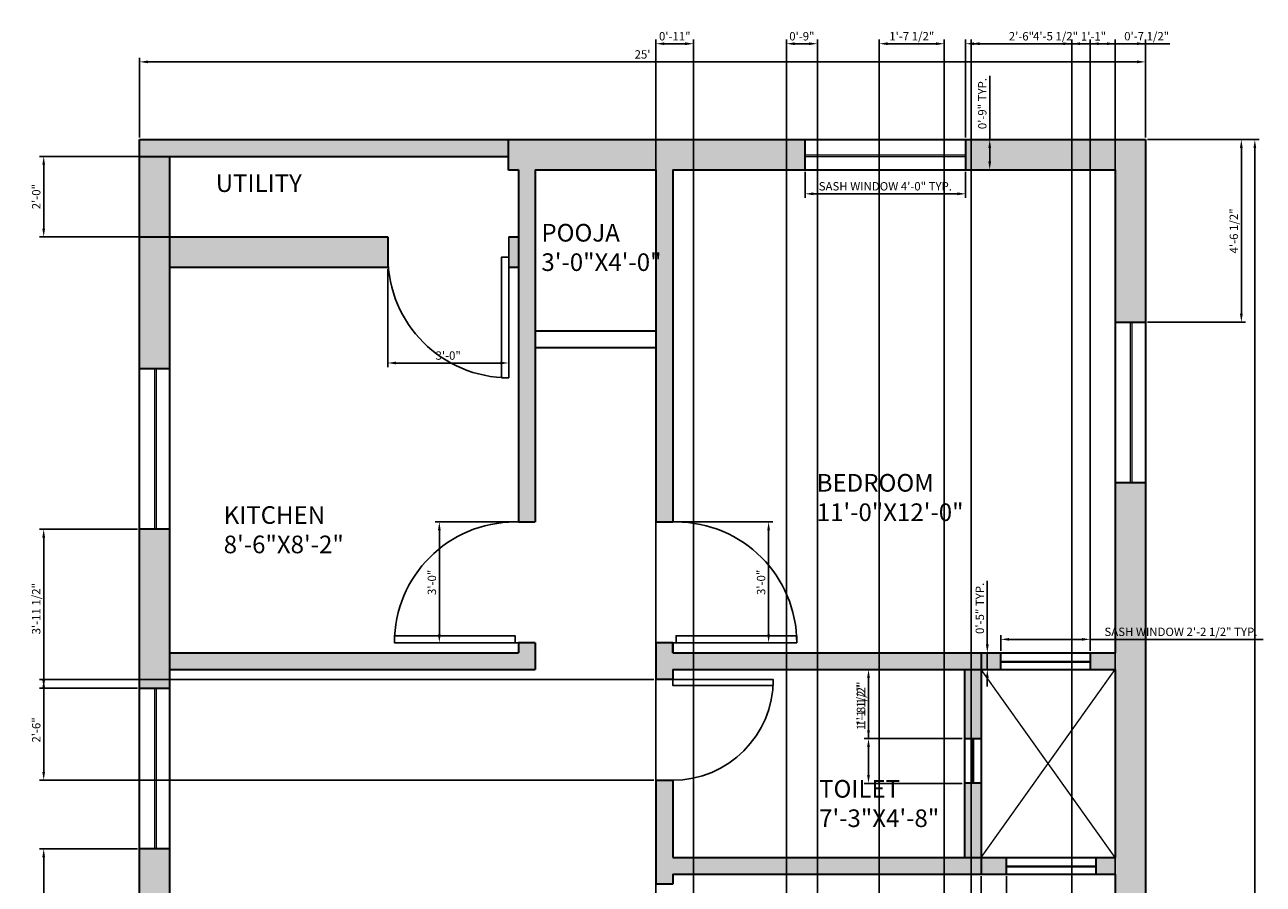
# Model space of a CAD drawing. Units: inches. Extents: x 2545 to 2915, y 1754 to 2359.
# Tile 2 of 2: x 2545 to 2915, y 2103 to 2359. Entities that reach past the tile are written whole.
import ezdxf

# ---------------------------------------------------------------- set-up
doc = ezdxf.new("R2010")
doc.units = ezdxf.units.IN
for name, color, linetype, lineweight in [('A-ANNO-DIMS', 2, 'Continuous', 18), ('A-AREA-IDEN', 7, 'Continuous', 25), ('A-DOOR', 3, 'Continuous', 25), ('A-FLOR-OPEN', 8, 'Continuous', 18), ('A-GLAZ', 4, 'Continuous', 18), ('A-WALL', 7, 'Continuous', 35), ('A-WALL-PATT', 252, 'Continuous', 13)]:
    doc.layers.add(name, color=color, linetype=linetype, lineweight=lineweight)
doc.styles.get("Standard").update_dxf_attribs({"font": 'arial.ttf'})
doc.dimstyles.new('ISO-25', dxfattribs={"dimtxt": 2.5, "dimasz": 2.5, "dimexe": 1.25, "dimexo": 0.625, "dimtad": 1, "dimlunit": 4, "dimtxsty": 'Standard', "dimcen": 2.5, "dimadec": 0, "dimazin": 0, "dimtfac": 1, "dimtmove": 0, "dimatfit": 3, "dimfxl": 1, "dimarcsym": 0})

# ---------------------------------------------------------------- blocks, each defined once
blk = doc.blocks.new('*U2')
for p, q in [((0, 0), (0, -5)), ((30, 0), (30, -5))]:
    blk.add_line(p, q)
blk.add_lwpolyline([(0, 0), (0, 30), (1.75, 30), (1.75, 0)], close=True)
blk.add_arc((0, 0), 30, 0, 90)
blk = doc.blocks.new('*D3')
at = {"layer": 'A-ANNO-DIMS', "color": 0, "lineweight": -2, "transparency": 16777216}
for p, q in [((2579.4, 2325.37), (2579.4, 2349.18)), ((2581.9, 2347.93), (2876.9, 2347.93)), ((2879.4, 2325.37), (2879.4, 2349.18))]:
    blk.add_line(p, q, dxfattribs=at)
at = {"layer": 'A-ANNO-DIMS', "color": 0, "transparency": 16777216}
for points in [[(2581.9, 2348.34), (2581.9, 2347.51), (2579.4, 2347.93)], [(2876.9, 2348.34), (2876.9, 2347.51), (2879.4, 2347.93)]]:
    blk.add_solid(points, dxfattribs=at)
at = {"layer": 'Defpoints', "color": 0, "transparency": 16777216}
for p in [(2879.4, 2347.93), (2579.4, 2324.74), (2879.4, 2324.74)]:
    blk.add_point(p, dxfattribs=at)
at = {"layer": 'A-ANNO-DIMS', "color": 0, "transparency": 16777216, "insert": (2729.4, 2349.83), "char_height": 2.5, "attachment_point": 5}
blk.add_mtext("25'", dxfattribs=at)
blk = doc.blocks.new('*D4')
at = {"layer": 'A-ANNO-DIMS', "color": 0, "lineweight": -2, "transparency": 16777216}
for p, q in [((2880.02, 2324.74), (2913.27, 2324.74)), ((2912.02, 2322.24), (2912.02, 1787.24)), ((2880.02, 1784.74), (2913.27, 1784.74))]:
    blk.add_line(p, q, dxfattribs=at)
at = {"layer": 'A-ANNO-DIMS', "color": 0, "transparency": 16777216}
for points in [[(2911.6, 2322.24), (2912.44, 2322.24), (2912.02, 2324.74)], [(2911.6, 1787.24), (2912.44, 1787.24), (2912.02, 1784.74)]]:
    blk.add_solid(points, dxfattribs=at)
at = {"layer": 'Defpoints', "color": 0, "transparency": 16777216}
for p in [(2879.4, 2324.74), (2879.4, 1784.74), (2912.02, 1784.74)]:
    blk.add_point(p, dxfattribs=at)
at = {"layer": 'A-ANNO-DIMS', "color": 0, "transparency": 16777216, "insert": (2910.12, 2054.74), "char_height": 2.5, "attachment_point": 5, "rotation": 90}
blk.add_mtext("45'", dxfattribs=at)
blk = doc.blocks.new('WIN-SASH-48')
for p, q in [((0, 8.97), (47.9, 8.97)), ((0, 4.48), (47.9, 4.48)), ((0, 3.98), (47.9, 3.98)), ((47.9, 0), (0, 0))]:
    blk.add_line(p, q)
blk = doc.blocks.new('WIN-SASH-26_71')
for p, q in [((0, 5), (26.71, 5)), ((0, 2.5), (26.71, 2.5)), ((0, 2.22), (26.71, 2.22)), ((26.71, 0), (0, 0))]:
    blk.add_line(p, q)
blk = doc.blocks.new('*D9')
at = {"layer": 'A-ANNO-DIMS', "color": 0, "lineweight": -2, "transparency": 16777216}
for p, q in [((2777.87, 2315.15), (2777.87, 2307.34)), ((2825.77, 2315.15), (2825.77, 2307.34)), ((2780.37, 2308.59), (2823.27, 2308.59))]:
    blk.add_line(p, q, dxfattribs=at)
at = {"layer": 'A-ANNO-DIMS', "color": 0, "transparency": 16777216}
for points in [[(2780.37, 2309.01), (2780.37, 2308.17), (2777.87, 2308.59)], [(2823.27, 2309.01), (2823.27, 2308.17), (2825.77, 2308.59)]]:
    blk.add_solid(points, dxfattribs=at)
at = {"layer": 'Defpoints', "color": 0, "transparency": 16777216}
for p in [(2777.87, 2315.78), (2825.77, 2315.78), (2825.77, 2308.59)]:
    blk.add_point(p, dxfattribs=at)
at = {"layer": 'A-ANNO-DIMS', "color": 0, "transparency": 16777216, "insert": (2801.82, 2310.51), "char_height": 2.5, "attachment_point": 5}
blk.add_mtext('SASH WINDOW 4\'-0" TYP.', dxfattribs=at)
blk = doc.blocks.new('*D10')
at = {"layer": 'A-ANNO-DIMS', "color": 0, "lineweight": -2, "transparency": 16777216}
for p, q in [((2832.95, 2324.74), (2832.95, 2343.73)), ((2826.39, 2324.74), (2834.2, 2324.74)), ((2832.95, 2318.28), (2832.95, 2322.24)), ((2826.39, 2315.78), (2834.2, 2315.78))]:
    blk.add_line(p, q, dxfattribs=at)
at = {"layer": 'A-ANNO-DIMS', "color": 0, "transparency": 16777216}
for points in [[(2832.54, 2322.24), (2833.37, 2322.24), (2832.95, 2324.74)], [(2832.54, 2318.28), (2833.37, 2318.28), (2832.95, 2315.78)]]:
    blk.add_solid(points, dxfattribs=at)
at = {"layer": 'Defpoints', "color": 0, "transparency": 16777216}
for p in [(2825.77, 2324.74), (2832.95, 2324.74), (2825.77, 2315.78)]:
    blk.add_point(p, dxfattribs=at)
at = {"layer": 'A-ANNO-DIMS', "color": 0, "transparency": 16777216, "insert": (2831.05, 2335.49), "char_height": 2.5, "attachment_point": 5, "rotation": 90}
blk.add_mtext('0\'-9" TYP.', dxfattribs=at)
blk = doc.blocks.new('*D11')
at = {"layer": 'A-ANNO-DIMS', "color": 0, "lineweight": -2, "transparency": 16777216}
for p, q in [((2836.23, 2172.37), (2836.23, 2177)), ((2838.73, 2175.75), (2860.44, 2175.75)), ((2862.94, 2172.37), (2862.94, 2177)), ((2862.94, 2175.75), (2914.52, 2175.75))]:
    blk.add_line(p, q, dxfattribs=at)
at = {"layer": 'A-ANNO-DIMS', "color": 0, "transparency": 16777216}
for points in [[(2838.73, 2176.16), (2838.73, 2175.33), (2836.23, 2175.75)], [(2860.44, 2176.16), (2860.44, 2175.33), (2862.94, 2175.75)]]:
    blk.add_solid(points, dxfattribs=at)
at = {"layer": 'Defpoints', "color": 0, "transparency": 16777216}
for p in [(2862.94, 2175.75), (2836.23, 2171.74), (2862.94, 2171.74)]:
    blk.add_point(p, dxfattribs=at)
at = {"layer": 'A-ANNO-DIMS', "color": 0, "transparency": 16777216, "insert": (2889.98, 2177.67), "char_height": 2.5, "attachment_point": 5}
blk.add_mtext('SASH WINDOW 2\'-2 1/2" TYP.', dxfattribs=at)
blk = doc.blocks.new('*D12')
at = {"layer": 'A-ANNO-DIMS', "color": 0, "lineweight": -2, "transparency": 16777216}
for p, q in [((2832.23, 2174.24), (2832.23, 2193.23)), ((2835.61, 2171.74), (2830.98, 2171.74)), ((2832.23, 2166.74), (2832.23, 2171.74)), ((2835.61, 2166.74), (2830.98, 2166.74)), ((2832.23, 2164.24), (2832.23, 2161.74))]:
    blk.add_line(p, q, dxfattribs=at)
at = {"layer": 'A-ANNO-DIMS', "color": 0, "transparency": 16777216}
for points in [[(2831.81, 2174.24), (2832.64, 2174.24), (2832.23, 2171.74)], [(2831.81, 2164.24), (2832.64, 2164.24), (2832.23, 2166.74)]]:
    blk.add_solid(points, dxfattribs=at)
at = {"layer": 'Defpoints', "color": 0, "transparency": 16777216}
for p in [(2832.23, 2171.74), (2836.23, 2171.74), (2836.23, 2166.74)]:
    blk.add_point(p, dxfattribs=at)
at = {"layer": 'A-ANNO-DIMS', "color": 0, "transparency": 16777216, "insert": (2830.32, 2184.99), "char_height": 2.5, "attachment_point": 5, "rotation": 90}
blk.add_mtext('0\'-5" TYP.', dxfattribs=at)
blk = doc.blocks.new('*D15')
at = {"layer": 'A-ANNO-DIMS', "color": 0, "lineweight": -2, "transparency": 16777216}
for p, q in [((2578.81, 2113.29), (2549.55, 2113.29)), ((2550.8, 2055.24), (2550.8, 2110.79)), ((2578.81, 2052.74), (2549.55, 2052.74))]:
    blk.add_line(p, q, dxfattribs=at)
at = {"layer": 'A-ANNO-DIMS', "color": 0, "transparency": 16777216}
for points in [[(2550.38, 2110.79), (2551.21, 2110.79), (2550.8, 2113.29)], [(2550.38, 2055.24), (2551.21, 2055.24), (2550.8, 2052.74)]]:
    blk.add_solid(points, dxfattribs=at)
at = {"layer": 'Defpoints', "color": 0, "transparency": 16777216}
for p in [(2550.8, 2113.29), (2579.43, 2113.29), (2579.43, 2052.74)]:
    blk.add_point(p, dxfattribs=at)
at = {"layer": 'A-ANNO-DIMS', "color": 0, "transparency": 16777216, "insert": (2548.88, 2083.01), "char_height": 2.5, "attachment_point": 5, "rotation": 90}
blk.add_mtext('5\'-0 1/2"', dxfattribs=at)
blk = doc.blocks.new('*D16')
at = {"layer": 'A-ANNO-DIMS', "color": 0, "lineweight": -2, "transparency": 16777216}
for p, q in [((2578.81, 2208.6), (2549.55, 2208.6)), ((2550.8, 2163.68), (2550.8, 2206.1)), ((2578.81, 2161.18), (2549.55, 2161.18))]:
    blk.add_line(p, q, dxfattribs=at)
at = {"layer": 'A-ANNO-DIMS', "color": 0, "transparency": 16777216}
for points in [[(2550.38, 2206.1), (2551.21, 2206.1), (2550.8, 2208.6)], [(2550.38, 2163.68), (2551.21, 2163.68), (2550.8, 2161.18)]]:
    blk.add_solid(points, dxfattribs=at)
at = {"layer": 'Defpoints', "color": 0, "transparency": 16777216}
for p in [(2550.8, 2208.6), (2579.43, 2208.6), (2579.43, 2161.18)]:
    blk.add_point(p, dxfattribs=at)
at = {"layer": 'A-ANNO-DIMS', "color": 0, "transparency": 16777216, "insert": (2548.88, 2184.89), "char_height": 2.5, "attachment_point": 5, "rotation": 90}
blk.add_mtext('3\'-11 1/2"', dxfattribs=at)
blk = doc.blocks.new('*D17')
at = {"layer": 'A-ANNO-DIMS', "color": 0, "lineweight": -2, "transparency": 16777216}
for p, q in [((2880.02, 2324.74), (2909.25, 2324.74)), ((2908, 2322.24), (2908, 2272.83)), ((2880.02, 2270.33), (2909.25, 2270.33))]:
    blk.add_line(p, q, dxfattribs=at)
at = {"layer": 'A-ANNO-DIMS', "color": 0, "transparency": 16777216}
for points in [[(2907.58, 2322.24), (2908.41, 2322.24), (2908, 2324.74)], [(2907.58, 2272.83), (2908.41, 2272.83), (2908, 2270.33)]]:
    blk.add_solid(points, dxfattribs=at)
at = {"layer": 'Defpoints', "color": 0, "transparency": 16777216}
for p in [(2879.4, 2324.74), (2879.4, 2270.33), (2908, 2270.33)]:
    blk.add_point(p, dxfattribs=at)
at = {"layer": 'A-ANNO-DIMS', "color": 0, "transparency": 16777216, "insert": (2906.08, 2297.53), "char_height": 2.5, "attachment_point": 5, "rotation": 90}
blk.add_mtext('4\'-6 1/2"', dxfattribs=at)
blk = doc.blocks.new('*D19')
at = {"layer": 'A-ANNO-DIMS', "color": 0, "lineweight": -2, "transparency": 16777216}
for p, q in [((2825.77, 2325.37), (2825.77, 2354.59)), ((2828.27, 2353.34), (2876.9, 2353.34)), ((2879.4, 2325.37), (2879.4, 2354.59))]:
    blk.add_line(p, q, dxfattribs=at)
at = {"layer": 'A-ANNO-DIMS', "color": 0, "transparency": 16777216}
for points in [[(2828.27, 2353.76), (2828.27, 2352.92), (2825.77, 2353.34)], [(2876.9, 2353.76), (2876.9, 2352.92), (2879.4, 2353.34)]]:
    blk.add_solid(points, dxfattribs=at)
at = {"layer": 'Defpoints', "color": 0, "transparency": 16777216}
for p in [(2879.4, 2353.34), (2825.77, 2324.74), (2879.4, 2324.74)]:
    blk.add_point(p, dxfattribs=at)
at = {"layer": 'A-ANNO-DIMS', "color": 0, "transparency": 16777216, "insert": (2852.58, 2355.26), "char_height": 2.5, "attachment_point": 5}
blk.add_mtext('4\'-5 1/2"', dxfattribs=at)
blk = doc.blocks.new('*D20')
at = {"layer": 'A-ANNO-DIMS', "color": 0, "lineweight": -2, "transparency": 16777216}
for p, q in [((2587.77, 2319.74), (2549.55, 2319.74)), ((2550.8, 2317.24), (2550.8, 2298.24)), ((2652.77, 2295.74), (2549.55, 2295.74))]:
    blk.add_line(p, q, dxfattribs=at)
at = {"layer": 'A-ANNO-DIMS', "color": 0, "transparency": 16777216}
for points in [[(2550.38, 2317.24), (2551.21, 2317.24), (2550.8, 2319.74)], [(2550.38, 2298.24), (2551.21, 2298.24), (2550.8, 2295.74)]]:
    blk.add_solid(points, dxfattribs=at)
at = {"layer": 'Defpoints', "color": 0, "transparency": 16777216}
for p in [(2588.4, 2319.74), (2550.8, 2295.74), (2653.4, 2295.74)]:
    blk.add_point(p, dxfattribs=at)
at = {"layer": 'A-ANNO-DIMS', "color": 0, "transparency": 16777216, "insert": (2548.89, 2307.74), "char_height": 2.5, "attachment_point": 5, "rotation": 90}
blk.add_mtext('2\'-0"', dxfattribs=at)
blk = doc.blocks.new('*D22')
at = {"layer": 'A-ANNO-DIMS', "color": 0, "lineweight": -2, "transparency": 16777216}
for p, q in [((2696.77, 2210.74), (2667.55, 2210.74)), ((2668.8, 2177.24), (2668.8, 2208.24)), ((2696.77, 2174.74), (2667.55, 2174.74))]:
    blk.add_line(p, q, dxfattribs=at)
at = {"layer": 'A-ANNO-DIMS', "color": 0, "transparency": 16777216}
for points in [[(2668.38, 2208.24), (2669.21, 2208.24), (2668.8, 2210.74)], [(2668.38, 2177.24), (2669.21, 2177.24), (2668.8, 2174.74)]]:
    blk.add_solid(points, dxfattribs=at)
at = {"layer": 'Defpoints', "color": 0, "transparency": 16777216}
for p in [(2668.8, 2210.74), (2697.4, 2210.74), (2697.4, 2174.74)]:
    blk.add_point(p, dxfattribs=at)
at = {"layer": 'A-ANNO-DIMS', "color": 0, "transparency": 16777216, "insert": (2666.89, 2192.74), "char_height": 2.5, "attachment_point": 5, "rotation": 90}
blk.add_mtext('3\'-0"', dxfattribs=at)
blk = doc.blocks.new('*D23')
at = {"layer": 'A-ANNO-DIMS', "color": 0, "lineweight": -2, "transparency": 16777216}
for p, q in [((2739.02, 2210.74), (2768.25, 2210.74)), ((2767, 2208.24), (2767, 2177.24)), ((2739.02, 2174.74), (2768.25, 2174.74))]:
    blk.add_line(p, q, dxfattribs=at)
at = {"layer": 'A-ANNO-DIMS', "color": 0, "transparency": 16777216}
for points in [[(2766.58, 2208.24), (2767.41, 2208.24), (2767, 2210.74)], [(2766.58, 2177.24), (2767.41, 2177.24), (2767, 2174.74)]]:
    blk.add_solid(points, dxfattribs=at)
at = {"layer": 'Defpoints', "color": 0, "transparency": 16777216}
for p in [(2738.4, 2210.74), (2738.4, 2174.74), (2767, 2174.74)]:
    blk.add_point(p, dxfattribs=at)
at = {"layer": 'A-ANNO-DIMS', "color": 0, "transparency": 16777216, "insert": (2765.09, 2192.74), "char_height": 2.5, "attachment_point": 5, "rotation": 90}
blk.add_mtext('3\'-0"', dxfattribs=at)
blk = doc.blocks.new('*D25')
at = {"layer": 'A-ANNO-DIMS', "color": 0, "lineweight": -2, "transparency": 16777216}
for p, q in [((2653.4, 2286.12), (2653.4, 2256.89)), ((2689.48, 2286.12), (2689.48, 2256.89)), ((2686.98, 2258.14), (2655.9, 2258.14))]:
    blk.add_line(p, q, dxfattribs=at)
at = {"layer": 'A-ANNO-DIMS', "color": 0, "transparency": 16777216}
for points in [[(2655.9, 2258.56), (2655.9, 2257.72), (2653.4, 2258.14)], [(2686.98, 2258.56), (2686.98, 2257.72), (2689.48, 2258.14)]]:
    blk.add_solid(points, dxfattribs=at)
at = {"layer": 'Defpoints', "color": 0, "transparency": 16777216}
for p in [(2653.4, 2286.74), (2689.48, 2286.74), (2653.4, 2258.14)]:
    blk.add_point(p, dxfattribs=at)
at = {"layer": 'A-ANNO-DIMS', "color": 0, "transparency": 16777216, "insert": (2671.44, 2260.04), "char_height": 2.5, "attachment_point": 5}
blk.add_mtext('3\'-0"', dxfattribs=at)
blk = doc.blocks.new('*D29')
at = {"layer": 'A-ANNO-DIMS', "color": 0, "lineweight": -2, "transparency": 16777216}
for p, q in [((2827.4, 1962.37), (2827.4, 2354.59)), ((2829.9, 2353.34), (2854.9, 2353.34)), ((2857.4, 1962.37), (2857.4, 2354.59))]:
    blk.add_line(p, q, dxfattribs=at)
at = {"layer": 'A-ANNO-DIMS', "color": 0, "transparency": 16777216}
for points in [[(2829.9, 2353.76), (2829.9, 2352.92), (2827.4, 2353.34)], [(2854.9, 2353.76), (2854.9, 2352.92), (2857.4, 2353.34)]]:
    blk.add_solid(points, dxfattribs=at)
at = {"layer": 'Defpoints', "color": 0, "transparency": 16777216}
for p in [(2857.4, 2353.34), (2827.4, 1961.74), (2857.4, 1961.74)]:
    blk.add_point(p, dxfattribs=at)
at = {"layer": 'A-ANNO-DIMS', "color": 0, "transparency": 16777216, "insert": (2842.4, 2355.24), "char_height": 2.5, "attachment_point": 5}
blk.add_mtext('2\'-6"', dxfattribs=at)
blk = doc.blocks.new('*D30')
at = {"layer": 'A-ANNO-DIMS', "color": 0, "lineweight": -2, "transparency": 16777216}
for p, q in [((2857.4, 1962.37), (2857.4, 2354.59)), ((2859.9, 2353.34), (2867.9, 2353.34)), ((2870.4, 1962.37), (2870.4, 2354.59))]:
    blk.add_line(p, q, dxfattribs=at)
at = {"layer": 'A-ANNO-DIMS', "color": 0, "transparency": 16777216}
for points in [[(2859.9, 2353.76), (2859.9, 2352.92), (2857.4, 2353.34)], [(2867.9, 2353.76), (2867.9, 2352.92), (2870.4, 2353.34)]]:
    blk.add_solid(points, dxfattribs=at)
at = {"layer": 'Defpoints', "color": 0, "transparency": 16777216}
for p in [(2870.4, 2353.34), (2857.4, 1961.74), (2870.4, 1961.74)]:
    blk.add_point(p, dxfattribs=at)
at = {"layer": 'A-ANNO-DIMS', "color": 0, "transparency": 16777216, "insert": (2863.9, 2355.22), "char_height": 2.5, "attachment_point": 5}
blk.add_mtext('1\'-1"', dxfattribs=at)
blk = doc.blocks.new('*D31')
at = {"layer": 'A-ANNO-DIMS', "color": 0, "lineweight": -2, "transparency": 16777216}
for p, q in [((2772.31, 1957.37), (2772.31, 2354.59)), ((2774.81, 2353.34), (2779.04, 2353.34)), ((2781.54, 1957.37), (2781.54, 2354.59))]:
    blk.add_line(p, q, dxfattribs=at)
at = {"layer": 'A-ANNO-DIMS', "color": 0, "transparency": 16777216}
for points in [[(2774.81, 2353.76), (2774.81, 2352.92), (2772.31, 2353.34)], [(2779.04, 2353.76), (2779.04, 2352.92), (2781.54, 2353.34)]]:
    blk.add_solid(points, dxfattribs=at)
at = {"layer": 'Defpoints', "color": 0, "transparency": 16777216}
for p in [(2781.54, 2353.34), (2772.31, 1956.74), (2781.54, 1956.74)]:
    blk.add_point(p, dxfattribs=at)
at = {"layer": 'A-ANNO-DIMS', "color": 0, "transparency": 16777216, "insert": (2776.92, 2355.24), "char_height": 2.5, "attachment_point": 5}
blk.add_mtext('0\'-9"', dxfattribs=at)
blk = doc.blocks.new('*D32')
at = {"layer": 'A-ANNO-DIMS', "color": 0, "lineweight": -2, "transparency": 16777216}
for p, q in [((2800, 1957.37), (2800, 2354.59)), ((2802.5, 2353.34), (2816.9, 2353.34)), ((2819.4, 1957.37), (2819.4, 2354.59))]:
    blk.add_line(p, q, dxfattribs=at)
at = {"layer": 'A-ANNO-DIMS', "color": 0, "transparency": 16777216}
for points in [[(2802.5, 2353.76), (2802.5, 2352.92), (2800, 2353.34)], [(2816.9, 2353.76), (2816.9, 2352.92), (2819.4, 2353.34)]]:
    blk.add_solid(points, dxfattribs=at)
at = {"layer": 'Defpoints', "color": 0, "transparency": 16777216}
for p in [(2819.4, 2353.34), (2800, 1956.74), (2819.4, 1956.74)]:
    blk.add_point(p, dxfattribs=at)
at = {"layer": 'A-ANNO-DIMS', "color": 0, "transparency": 16777216, "insert": (2809.7, 2355.26), "char_height": 2.5, "attachment_point": 5}
blk.add_mtext('1\'-7 1/2"', dxfattribs=at)
blk = doc.blocks.new('*D35')
at = {"layer": 'A-ANNO-DIMS', "color": 0, "lineweight": -2, "transparency": 16777216}
for p, q in [((2733.4, 1957.37), (2733.4, 2354.59)), ((2735.9, 2353.34), (2742.11, 2353.34)), ((2744.61, 1957.37), (2744.61, 2354.59))]:
    blk.add_line(p, q, dxfattribs=at)
at = {"layer": 'A-ANNO-DIMS', "color": 0, "transparency": 16777216}
for points in [[(2735.9, 2353.76), (2735.9, 2352.92), (2733.4, 2353.34)], [(2742.11, 2353.76), (2742.11, 2352.92), (2744.61, 2353.34)]]:
    blk.add_solid(points, dxfattribs=at)
at = {"layer": 'Defpoints', "color": 0, "transparency": 16777216}
for p in [(2744.61, 2353.34), (2733.4, 1956.74), (2744.61, 1956.74)]:
    blk.add_point(p, dxfattribs=at)
at = {"layer": 'A-ANNO-DIMS', "color": 0, "transparency": 16777216, "insert": (2739.01, 2355.24), "char_height": 2.5, "attachment_point": 5}
blk.add_mtext('0\'-11"', dxfattribs=at)
blk = doc.blocks.new('*D38')
at = {"layer": 'A-ANNO-DIMS', "color": 0, "lineweight": -2, "transparency": 16777216}
for p, q in [((2796.8, 2146.15), (2796.8, 2162.14)), ((2824.77, 2146.15), (2795.55, 2146.15)), ((2796.8, 2135.32), (2796.8, 2143.65)), ((2824.77, 2132.82), (2795.55, 2132.82))]:
    blk.add_line(p, q, dxfattribs=at)
at = {"layer": 'A-ANNO-DIMS', "color": 0, "transparency": 16777216}
for points in [[(2796.38, 2143.65), (2797.21, 2143.65), (2796.8, 2146.15)], [(2796.38, 2135.32), (2797.21, 2135.32), (2796.8, 2132.82)]]:
    blk.add_solid(points, dxfattribs=at)
at = {"layer": 'Defpoints', "color": 0, "transparency": 16777216}
for p in [(2796.8, 2146.15), (2825.4, 2146.15), (2825.4, 2132.82)]:
    blk.add_point(p, dxfattribs=at)
at = {"layer": 'A-ANNO-DIMS', "color": 0, "transparency": 16777216, "insert": (2794.88, 2155.39), "char_height": 2.5, "attachment_point": 5, "rotation": 90}
blk.add_mtext('1\'-1 1/2"', dxfattribs=at)
blk = doc.blocks.new('*D39')
at = {"layer": 'A-ANNO-DIMS', "color": 0, "lineweight": -2, "transparency": 16777216}
for p, q in [((2824.77, 2166.74), (2795.55, 2166.74)), ((2796.8, 2148.65), (2796.8, 2164.24)), ((2824.77, 2146.15), (2795.55, 2146.15))]:
    blk.add_line(p, q, dxfattribs=at)
at = {"layer": 'A-ANNO-DIMS', "color": 0, "transparency": 16777216}
for points in [[(2796.38, 2164.24), (2797.21, 2164.24), (2796.8, 2166.74)], [(2796.38, 2148.65), (2797.21, 2148.65), (2796.8, 2146.15)]]:
    blk.add_solid(points, dxfattribs=at)
at = {"layer": 'Defpoints', "color": 0, "transparency": 16777216}
for p in [(2796.8, 2166.74), (2825.4, 2166.74), (2825.4, 2146.15)]:
    blk.add_point(p, dxfattribs=at)
at = {"layer": 'A-ANNO-DIMS', "color": 0, "transparency": 16777216, "insert": (2794.88, 2156.45), "char_height": 2.5, "attachment_point": 5, "rotation": 90}
blk.add_mtext('1\'-8 1/2"', dxfattribs=at)
blk = doc.blocks.new('*D40')
at = {"layer": 'A-ANNO-DIMS', "color": 0, "lineweight": -2, "transparency": 16777216}
for p, q in [((2862.94, 2172.37), (2862.94, 2354.59)), ((2865.44, 2353.34), (2867.9, 2353.34)), ((2870.4, 2172.37), (2870.4, 2354.59)), ((2870.4, 2353.34), (2886.62, 2353.34))]:
    blk.add_line(p, q, dxfattribs=at)
at = {"layer": 'A-ANNO-DIMS', "color": 0, "transparency": 16777216}
for points in [[(2865.44, 2353.76), (2865.44, 2352.92), (2862.94, 2353.34)], [(2867.9, 2353.76), (2867.9, 2352.92), (2870.4, 2353.34)]]:
    blk.add_solid(points, dxfattribs=at)
at = {"layer": 'Defpoints', "color": 0, "transparency": 16777216}
for p in [(2870.4, 2353.34), (2862.94, 2171.74), (2870.4, 2171.74)]:
    blk.add_point(p, dxfattribs=at)
at = {"layer": 'A-ANNO-DIMS', "color": 0, "transparency": 16777216, "insert": (2879.76, 2355.26), "char_height": 2.5, "attachment_point": 5}
blk.add_mtext('0\'-7 1/2"', dxfattribs=at)
blk = doc.blocks.new('*D41')
at = {"layer": 'A-ANNO-DIMS', "color": 0, "lineweight": -2, "transparency": 16777216}
for p, q in [((2830.4, 2105.12), (2830.4, 1754.89)), ((2837.91, 2105.12), (2837.91, 1754.89)), ((2830.4, 1756.14), (2814.17, 1756.14)), ((2835.41, 1756.14), (2832.9, 1756.14))]:
    blk.add_line(p, q, dxfattribs=at)
at = {"layer": 'A-ANNO-DIMS', "color": 0, "transparency": 16777216}
for points in [[(2832.9, 1756.56), (2832.9, 1755.72), (2830.4, 1756.14)], [(2835.41, 1756.56), (2835.41, 1755.72), (2837.91, 1756.14)]]:
    blk.add_solid(points, dxfattribs=at)
at = {"layer": 'Defpoints', "color": 0, "transparency": 16777216}
for p in [(2830.4, 2105.74), (2837.91, 2105.74), (2830.4, 1756.14)]:
    blk.add_point(p, dxfattribs=at)
at = {"layer": 'A-ANNO-DIMS', "color": 0, "transparency": 16777216, "insert": (2821.04, 1758.06), "char_height": 2.5, "attachment_point": 5}
blk.add_mtext('0\'-7 1/2"', dxfattribs=at)
blk = doc.blocks.new('*D42')
at = {"layer": 'A-ANNO-DIMS', "color": 0, "lineweight": -2, "transparency": 16777216}
for p, q in [((2732.77, 2163.74), (2549.55, 2163.74)), ((2550.8, 2161.24), (2550.8, 2136.24)), ((2732.77, 2133.74), (2549.55, 2133.74))]:
    blk.add_line(p, q, dxfattribs=at)
at = {"layer": 'A-ANNO-DIMS', "color": 0, "transparency": 16777216}
for points in [[(2550.38, 2161.24), (2551.21, 2161.24), (2550.8, 2163.74)], [(2550.38, 2136.24), (2551.21, 2136.24), (2550.8, 2133.74)]]:
    blk.add_solid(points, dxfattribs=at)
at = {"layer": 'Defpoints', "color": 0, "transparency": 16777216}
for p in [(2733.4, 2163.74), (2550.8, 2133.74), (2733.4, 2133.74)]:
    blk.add_point(p, dxfattribs=at)
at = {"layer": 'A-ANNO-DIMS', "color": 0, "transparency": 16777216, "insert": (2548.89, 2148.74), "char_height": 2.5, "attachment_point": 5, "rotation": 90}
blk.add_mtext('2\'-6"', dxfattribs=at)
blk = doc.blocks.new('*D43')
at = {"layer": 'A-ANNO-DIMS', "color": 0, "lineweight": -2, "transparency": 16777216}
for p, q in [((2830.4, 2105.12), (2830.4, 1754.89)), ((2870.4, 2105.12), (2870.4, 1754.89)), ((2832.9, 1756.14), (2867.9, 1756.14))]:
    blk.add_line(p, q, dxfattribs=at)
at = {"layer": 'A-ANNO-DIMS', "color": 0, "transparency": 16777216}
for points in [[(2832.9, 1756.56), (2832.9, 1755.72), (2830.4, 1756.14)], [(2867.9, 1756.56), (2867.9, 1755.72), (2870.4, 1756.14)]]:
    blk.add_solid(points, dxfattribs=at)
at = {"layer": 'Defpoints', "color": 0, "transparency": 16777216}
for p in [(2830.4, 2105.74), (2870.4, 2105.74), (2870.4, 1756.14)]:
    blk.add_point(p, dxfattribs=at)
at = {"layer": 'A-ANNO-DIMS', "color": 0, "transparency": 16777216, "insert": (2850.4, 1758.04), "char_height": 2.5, "attachment_point": 5}
blk.add_mtext('3\'-4"', dxfattribs=at)

msp = doc.modelspace()

# ---------------------------------------------------------------- hatches: boundary and pattern name
at = {"layer": 'A-WALL-PATT'}
h = msp.add_hatch(color=256, dxfattribs=at)
h.dxf.hatch_style = 1
h.paths.add_polyline_path([(2689.398, 2319.741), (2689.398, 2324.741), (2579.396, 2324.741), (2579.396, 2319.741)])
h = msp.add_hatch(color=256, dxfattribs=at)
h.dxf.hatch_style = 1
h.paths.add_polyline_path([(2777.87, 2324.741), (2689.398, 2324.741), (2689.398, 2315.741), (2692.396, 2315.741), (2692.396, 2210.741), (2697.396, 2210.741), (2697.396, 2315.741), (2733.396, 2315.741), (2733.396, 2210.741), (2738.396, 2210.741), (2738.396, 2315.741), (2777.87, 2315.741)])
h = msp.add_hatch(color=256, dxfattribs=at)
h.dxf.hatch_style = 1
h.paths.add_polyline_path([(2879.396, 2324.741), (2825.768, 2324.741), (2825.768, 2315.741), (2870.396, 2315.741), (2870.396, 2270.328), (2879.396, 2270.328)])
h = msp.add_hatch(color=256, dxfattribs=at)
h.dxf.hatch_style = 1
h.paths.add_polyline_path([(2588.396, 2319.741), (2579.396, 2319.741), (2579.396, 2295.741), (2588.396, 2295.741)])
h = msp.add_hatch(color=256, dxfattribs=at)
h.dxf.hatch_style = 1
h.paths.add_polyline_path([(2588.396, 2295.741), (2579.396, 2295.741), (2579.396, 2256.502), (2588.396, 2256.502)])
h = msp.add_hatch(color=256, dxfattribs=at)
h.dxf.hatch_style = 1
h.paths.add_polyline_path([(2653.398, 2295.741), (2588.396, 2295.741), (2588.396, 2286.741), (2653.398, 2286.741)])
h = msp.add_hatch(color=256, dxfattribs=at)
h.dxf.hatch_style = 1
h.paths.add_polyline_path([(2692.396, 2295.741), (2689.48, 2295.741), (2689.48, 2289.741), (2689.48, 2286.741), (2692.396, 2286.741)])
h = msp.add_hatch(color=256, dxfattribs=at)
h.dxf.hatch_style = 1
h.paths.add_polyline_path([(2879.396, 2222.429), (2870.396, 2222.429), (2870.396, 2171.741), (2862.945, 2171.741), (2862.945, 2166.741), (2870.396, 2166.741), (2870.396, 2110.741), (2864.62, 2110.741), (2864.62, 2105.741), (2870.396, 2105.741), (2870.396, 2057.805), (2879.396, 2057.805)])
h = msp.add_hatch(color=256, dxfattribs=at)
h.dxf.hatch_style = 1
h.paths.add_polyline_path([(2588.396, 2208.604), (2579.396, 2208.604), (2579.396, 2161.184), (2588.396, 2161.184)])
h = msp.add_hatch(color=256, dxfattribs=at)
h.dxf.hatch_style = 1
h.paths.add_polyline_path([(2697.396, 2174.741), (2692.396, 2174.741), (2692.396, 2171.741), (2588.396, 2171.741), (2588.396, 2166.741), (2697.396, 2166.741)])
h = msp.add_hatch(color=256, dxfattribs=at)
h.dxf.hatch_style = 1
h.paths.add_polyline_path([(2830.396, 2171.741), (2738.396, 2171.741), (2738.396, 2174.741), (2733.396, 2174.741), (2733.396, 2163.741), (2738.396, 2163.741), (2738.396, 2166.741), (2830.396, 2166.741)])
h = msp.add_hatch(color=256, dxfattribs=at)
h.dxf.hatch_style = 1
h.paths.add_polyline_path([(2836.233, 2171.741), (2830.396, 2171.741), (2830.396, 2166.741), (2836.233, 2166.741)])
h = msp.add_hatch(color=256, dxfattribs=at)
h.dxf.hatch_style = 1
h.paths.add_polyline_path([(2830.396, 2166.741), (2825.396, 2166.741), (2825.396, 2146.151), (2830.396, 2146.151)])
h = msp.add_hatch(color=256, dxfattribs=at)
h.dxf.hatch_style = 1
h.paths.add_polyline_path([(2830.396, 2110.741), (2738.396, 2110.741), (2738.396, 2133.741), (2733.396, 2133.741), (2733.396, 2102.741), (2738.396, 2102.741), (2738.396, 2105.741), (2830.396, 2105.741)])
h = msp.add_hatch(color=256, dxfattribs=at)
h.dxf.hatch_style = 1
h.paths.add_polyline_path([(2830.396, 2132.823), (2825.396, 2132.823), (2825.396, 2110.741), (2830.396, 2110.741)], flags=17)
h = msp.add_hatch(color=256, dxfattribs=at)
h.dxf.hatch_style = 1
h.paths.add_polyline_path([(2588.396, 2113.285), (2579.396, 2113.285), (2579.396, 2052.737), (2588.396, 2052.737)])
h = msp.add_hatch(color=256, dxfattribs=at)
h.dxf.hatch_style = 1
h.paths.add_polyline_path([(2837.908, 2110.741), (2830.396, 2110.741), (2830.396, 2105.741), (2837.908, 2105.741)])

# ---------------------------------------------------------------- linework, layer by layer
at = {"layer": 'A-FLOR-OPEN'}
for p, q in [((2830.396, 2110.741), (2870.396, 2166.741)), ((2870.396, 2110.741), (2830.396, 2166.741))]:
    msp.add_line(p, q, dxfattribs=at)
at = {"layer": 'A-GLAZ'}
for p, q in [((2825.396, 2132.823), (2825.396, 2146.151)), ((2827.896, 2132.823), (2827.896, 2146.151)), ((2828.175, 2132.823), (2828.175, 2146.151)), ((2830.396, 2146.151), (2830.396, 2132.823))]:
    msp.add_line(p, q, dxfattribs=at)
at = {"layer": 'A-WALL'}
for p, q in [((2579.396, 1784.741), (2579.396, 2324.741)), ((2579.396, 2324.741), (2689.398, 2324.741)), ((2689.398, 2324.741), (2879.396, 2324.741)), ((2689.398, 2315.62), (2689.398, 2324.741)), ((2777.87, 2315.775), (2777.87, 2324.741)), ((2825.768, 2324.741), (2825.768, 2315.775)), ((2879.396, 2324.741), (2879.396, 1784.741)), ((2579.396, 2319.741), (2689.398, 2319.741)), ((2588.396, 1793.741), (2588.396, 2319.741)), ((2692.396, 2315.741), (2689.398, 2315.62)), ((2689.398, 2315.741), (2692.396, 2315.741)), ((2692.396, 2315.741), (2692.396, 2210.741)), ((2697.396, 2315.741), (2697.396, 2210.741)), ((2697.396, 2315.741), (2733.396, 2315.741)), ((2733.396, 2315.741), (2733.396, 2210.741)), ((2738.396, 2315.741), (2738.396, 2210.741)), ((2738.396, 2315.741), (2870.396, 2315.741)), ((2870.396, 2315.741), (2870.396, 2171.741)), ((2579.396, 2295.741), (2653.398, 2295.741)), ((2653.398, 2295.66), (2653.398, 2286.741)), ((2689.48, 2295.741), (2692.396, 2295.741)), ((2588.396, 2286.741), (2653.398, 2286.741)), ((2689.48, 2286.741), (2692.396, 2286.741)), ((2870.43, 2270.328), (2879.396, 2270.328)), ((2697.396, 2267.741), (2733.396, 2267.741)), ((2697.396, 2262.741), (2733.396, 2262.741)), ((2579.43, 2256.502), (2588.396, 2256.502)), ((2879.396, 2222.429), (2870.43, 2222.429)), ((2692.396, 2210.741), (2697.396, 2210.741)), ((2733.396, 2210.741), (2738.396, 2210.741)), ((2588.396, 2208.604), (2579.43, 2208.604)), ((2697.396, 2174.741), (2692.396, 2174.741)), ((2692.396, 2174.741), (2692.396, 2171.741)), ((2697.396, 2174.741), (2697.396, 2166.741)), ((2738.396, 2174.741), (2733.396, 2174.741)), ((2733.396, 2174.741), (2733.396, 2163.741)), ((2738.396, 2171.741), (2738.396, 2174.741)), ((2738.396, 2174.741), (2738.396, 2171.741)), ((2588.396, 2171.741), (2692.396, 2171.741)), ((2738.396, 2171.741), (2870.396, 2171.741)), ((2830.396, 2171.741), (2830.396, 2105.741)), ((2836.233, 2166.741), (2836.233, 2171.741)), ((2862.945, 2171.741), (2862.945, 2166.741)), ((2588.396, 2166.741), (2697.396, 2166.741)), ((2738.396, 2166.741), (2870.396, 2166.741)), ((2738.396, 2166.741), (2738.396, 2163.741)), ((2738.396, 2166.741), (2738.396, 2163.741)), ((2825.396, 2166.741), (2825.396, 2110.741)), ((2870.396, 2166.741), (2870.396, 2110.741)), ((2579.43, 2161.184), (2588.396, 2161.184)), ((2738.396, 2163.741), (2733.396, 2163.741)), ((2825.396, 2146.151), (2830.396, 2146.151)), ((2733.396, 2133.741), (2738.396, 2133.741)), ((2733.396, 2133.741), (2733.396, 2102.741)), ((2738.396, 2133.741), (2738.396, 2110.741)), ((2830.396, 2132.823), (2825.396, 2132.823)), ((2588.396, 2113.285), (2579.43, 2113.285)), ((2738.396, 2110.741), (2870.396, 2110.741)), ((2837.908, 2105.741), (2837.908, 2110.741)), ((2864.62, 2110.741), (2864.62, 2105.741)), ((2738.396, 2105.741), (2870.396, 2105.741)), ((2738.396, 2105.741), (2738.396, 2102.741)), ((2738.396, 2105.741), (2738.396, 2102.741)), ((2870.396, 2105.741), (2870.396, 1961.741)), ((2738.396, 2102.741), (2733.396, 2102.741))]:
    msp.add_line(p, q, dxfattribs=at)

# ---------------------------------------------------------------- block references
at = {"layer": 'A-DOOR', "yscale": 1.199999999999999, "zscale": 1.199999999999999}
for p, xscale, rotation in [((2689.48, 2289.741), 1.199999999999999, 180), ((2691.396, 2174.741), 1.199999999999999, 90), ((2739.396, 2174.741), -1.199999999999999, 270)]:
    msp.add_blockref('*U2', p, dxfattribs=dict(at, xscale=xscale, rotation=rotation))
at = {"layer": 'A-DOOR', "rotation": 270}
msp.add_blockref('*U2', (2738.396, 2163.741), dxfattribs=at)
at = {"layer": 'A-GLAZ'}
for name, p in [('WIN-SASH-48', (2777.87, 2315.775)), ('WIN-SASH-26_71', (2836.233, 2166.741)), ('WIN-SASH-26_71', (2837.908, 2105.741))]:
    msp.add_blockref(name, p, dxfattribs=at)
for p, rotation in [((2879.396, 2222.43), 90.0000000000021), ((2588.396, 2208.604), 90.00000000000087), ((2588.396, 2113.286), 90.00000000000087)]:
    msp.add_blockref('WIN-SASH-48', p, dxfattribs=dict(at, rotation=rotation))

# ---------------------------------------------------------------- texts
at = {"layer": 'A-AREA-IDEN', "attachment_point": 1}
for s, width, heights, insert, char_height in [('UTILITY', 4.6518, [0], (2602.103, 2314.391), 5.2603), ('POOJA\\P3\'-0"X4\'-0"', 5.26031, [14.236], (2699.238, 2299.609), 5.26031), ('BEDROOM\\P11\'-0"X12\'-0"', 4.6518, [0], (2781.348, 2225.051), 5.26031), ('KITCHEN\\P8\'-6"X8\'-2"', 4.6518, [0], (2604.478, 2215.447), 5.26031), ('TOILET\\P7\'-3"X4\'-8"', 4.6518, [0], (2782.063, 2133.816), 5.26031)]:
    msp.add_mtext_dynamic_manual_height_columns(s, width=width, gutter_width=26.302, heights=heights, dxfattribs=dict(at, insert=insert, char_height=char_height))

# ---------------------------------------------------------------- dimensions: what is measured, and where the dimension line sits
at = {"layer": 'A-ANNO-DIMS'}
for base, p1, p2, override, picture, middle in [((2744.614, 2353.341), (2733.396, 1956.741), (2744.614, 1956.741), {"dimdec": 1, "dimlfac": 1, "dimrnd": 0, "dimzin": 1, "dimdsep": 46, "dimlunit": 4, "dimfrac": 2}, '*D35', (2739.005, 2355.242)), ((2781.535, 2353.341), (2772.305, 1956.741), (2781.535, 1956.741), {"dimdec": 1, "dimlfac": 1, "dimrnd": 0, "dimzin": 1, "dimdsep": 46, "dimlunit": 4, "dimfrac": 2}, '*D31', (2776.92, 2355.242)), ((2819.396, 2353.341), (2799.996, 1956.741), (2819.396, 1956.741), {"dimdec": 1, "dimlfac": 1, "dimrnd": 0, "dimzin": 1, "dimdsep": 46, "dimlunit": 4, "dimfrac": 2}, '*D32', (2809.696, 2355.259)), ((2879.396, 2353.341), (2825.768, 2324.741), (2879.396, 2324.741), {"dimdec": 1, "dimlfac": 1, "dimrnd": 0, "dimzin": 1, "dimdsep": 46, "dimlunit": 4, "dimfrac": 2}, '*D19', (2852.582, 2355.259)), ((2857.396, 2353.341), (2827.396, 1961.741), (2857.396, 1961.741), {"dimdec": 1, "dimlfac": 1, "dimrnd": 0, "dimzin": 1, "dimdsep": 46, "dimlunit": 4, "dimfrac": 2}, '*D29', (2842.396, 2355.242)), ((2870.396, 2353.341), (2857.396, 1961.741), (2870.396, 1961.741), {"dimdec": 1, "dimlfac": 1, "dimrnd": 0, "dimzin": 1, "dimdsep": 46, "dimlunit": 4, "dimfrac": 2}, '*D30', (2863.896, 2355.221)), ((2870.396, 2353.341), (2862.945, 2171.741), (2870.396, 2171.741), {"dimdec": 1, "dimlfac": 1, "dimrnd": 0, "dimzin": 1, "dimdsep": 46, "dimlunit": 4, "dimfrac": 2}, '*D40', (2879.756, 2355.259)), ((2879.396, 2347.926), (2579.396, 2324.741), (2879.396, 2324.741), {"dimclrd": 0, "dimclre": 0, "dimclrt": 0}, '*D3', (2729.396, 2349.828)), ((2830.396, 1756.141), (2837.908, 2105.741), (2830.396, 2105.741), {"dimdec": 1, "dimlfac": 1, "dimrnd": 0, "dimzin": 1, "dimdsep": 46, "dimlunit": 4, "dimfrac": 2}, '*D41', (2821.035, 1758.059)), ((2870.396, 1756.141), (2830.396, 2105.741), (2870.396, 2105.741), {"dimdec": 1, "dimlfac": 1, "dimrnd": 0, "dimzin": 1, "dimdsep": 46, "dimlunit": 4, "dimfrac": 2}, '*D43', (2850.396, 1758.043))]:
    dim = msp.add_linear_dim(base=base, p1=p1, p2=p2, dimstyle='ISO-25', override=override, dxfattribs=at)
    dim.commit()
    dim.dimension.update_dxf_attribs({"geometry": picture, "text_midpoint": middle})
for base, p1, p2, picture, middle in [((2832.953, 2324.741), (2825.768, 2315.775), (2825.768, 2324.741), '*D10', (2831.052, 2335.485)), ((2832.226, 2171.741), (2836.233, 2166.741), (2836.233, 2171.741), '*D12', (2830.324, 2184.985))]:
    dim = msp.add_linear_dim(base=base, p1=p1, p2=p2, angle=90, text='<> TYP.', dimstyle='ISO-25', override={"dimdec": 1, "dimlfac": 1, "dimrnd": 0, "dimzin": 1, "dimdsep": 46, "dimlunit": 4, "dimfrac": 2}, dxfattribs=at)
    dim.commit()
    dim.dimension.update_dxf_attribs({"geometry": picture, "text_midpoint": middle})
for base, p1, p2, angle, override, picture, middle in [((2912.021, 1784.741), (2879.396, 2324.741), (2879.396, 1784.741), 90, {"dimclrd": 0, "dimclre": 0, "dimclrt": 0}, '*D4', (2910.125, 2054.741)), ((2907.996, 2270.328), (2879.396, 2324.741), (2879.396, 2270.328), 90, {"dimdec": 1, "dimlfac": 1, "dimrnd": 0, "dimzin": 1, "dimdsep": 46, "dimlunit": 4, "dimfrac": 2}, '*D17', (2906.078, 2297.535)), ((2550.796, 2295.741), (2588.396, 2319.741), (2653.398, 2295.741), 90, {"dimdec": 1, "dimlfac": 1, "dimrnd": 0, "dimzin": 1, "dimdsep": 46, "dimlunit": 4, "dimfrac": 2}, '*D20', (2548.894, 2307.741)), ((2653.398, 2258.141), (2689.48, 2286.741), (2653.398, 2286.741), 180, {"dimdec": 1, "dimlfac": 1, "dimrnd": 0, "dimzin": 1, "dimdsep": 46, "dimlunit": 4, "dimfrac": 2}, '*D25', (2671.439, 2260.043)), ((2668.796, 2210.741), (2697.396, 2174.741), (2697.396, 2210.741), 90, {"dimdec": 1, "dimlfac": 1, "dimrnd": 0, "dimzin": 1, "dimdsep": 46, "dimlunit": 4, "dimfrac": 2}, '*D22', (2666.894, 2192.741)), ((2766.996, 2174.741), (2738.396, 2210.741), (2738.396, 2174.741), 270, {"dimdec": 1, "dimlfac": 1, "dimrnd": 0, "dimzin": 1, "dimdsep": 46, "dimlunit": 4, "dimfrac": 2}, '*D23', (2765.094, 2192.741)), ((2550.796, 2208.604), (2579.43, 2161.184), (2579.43, 2208.604), 90, {"dimdec": 1, "dimlfac": 1, "dimrnd": 0, "dimzin": 1, "dimdsep": 46, "dimlunit": 4, "dimfrac": 2}, '*D16', (2548.877, 2184.894)), ((2796.796, 2166.741), (2825.396, 2146.151), (2825.396, 2166.741), 90, {"dimdec": 1, "dimlfac": 1, "dimrnd": 0, "dimzin": 1, "dimdsep": 46, "dimlunit": 4, "dimfrac": 2}, '*D39', (2794.878, 2156.446)), ((2550.796, 2133.741), (2733.396, 2163.741), (2733.396, 2133.741), 90, {"dimdec": 1, "dimlfac": 1, "dimrnd": 0, "dimzin": 1, "dimdsep": 46, "dimlunit": 4, "dimfrac": 2}, '*D42', (2548.894, 2148.741)), ((2796.796, 2146.151), (2825.396, 2132.823), (2825.396, 2146.151), 90, {"dimdec": 1, "dimlfac": 1, "dimrnd": 0, "dimzin": 1, "dimdsep": 46, "dimlunit": 4, "dimfrac": 2}, '*D38', (2794.878, 2155.394)), ((2550.796, 2113.285), (2579.43, 2052.737), (2579.43, 2113.285), 90, {"dimdec": 1, "dimlfac": 1, "dimrnd": 0, "dimzin": 1, "dimdsep": 46, "dimlunit": 4, "dimfrac": 2}, '*D15', (2548.878, 2083.011))]:
    dim = msp.add_linear_dim(base=base, p1=p1, p2=p2, angle=angle, dimstyle='ISO-25', override=override, dxfattribs=at)
    dim.commit()
    dim.dimension.update_dxf_attribs({"geometry": picture, "text_midpoint": middle})
for base, p1, p2, picture, middle in [((2825.768, 2308.59), (2777.87, 2315.775), (2825.768, 2315.775), '*D9', (2801.819, 2310.509)), ((2862.945, 2175.748), (2836.233, 2171.741), (2862.945, 2171.741), '*D11', (2889.983, 2177.666))]:
    dim = msp.add_linear_dim(base=base, p1=p1, p2=p2, text='SASH WINDOW <> TYP.', dimstyle='ISO-25', override={"dimdec": 1, "dimlfac": 1, "dimrnd": 0, "dimzin": 1, "dimdsep": 46, "dimlunit": 4, "dimfrac": 2}, dxfattribs=at)
    dim.commit()
    dim.dimension.update_dxf_attribs({"geometry": picture, "text_midpoint": middle})

doc.saveas('drawing.dxf')
